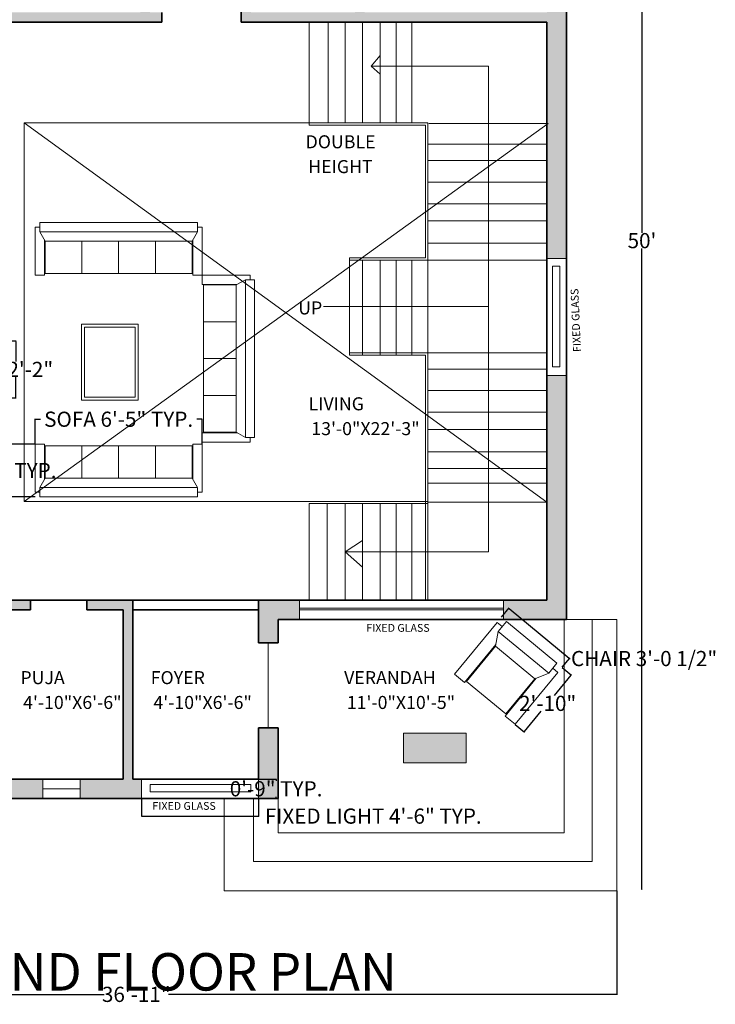
# Model space of a CAD drawing. Units: inches. Extents: x 136 to 672, y -412 to 279.
# Tile 3 of 6: x 351 to 672, y -412 to 42. Entities that reach past the tile are written whole.
import ezdxf

# ---------------------------------------------------------------- set-up
doc = ezdxf.new("R2010")
doc.units = ezdxf.units.IN
doc.header["$MEASUREMENT"] = 0
for name, color, linetype, lineweight in [('A-ANNO-DIMS', 12, 'Continuous', 18), ('A-ANNO-SYMB', 12, 'Continuous', 13), ('A-ANNO-TEXT', 7, 'Continuous', 18), ('A-AREA-IDEN', 7, 'Continuous', 18), ('A-DOOR', 4, 'Continuous', 18), ('A-FLOR-OPEN', 254, 'Continuous', 13), ('A-FLOR-STRS', 252, 'Continuous', 18), ('A-FURN-PATT', 143, 'Continuous', 9), ('A-WALL-PATT', 244, 'Continuous', 9), ('furniture', 252, 'Continuous', 18), ('walls', 253, 'Continuous', 35), ('windows', 171, 'Continuous', 18)]:
    doc.layers.add(name, color=color, linetype=linetype, lineweight=lineweight)
doc.styles.get("Standard").update_dxf_attribs({"font": 'arial.ttf'})
doc.dimstyles.get("Standard").update_dxf_attribs({"dimtxt": 7, "dimasz": 0.18, "dimexe": 0.18, "dimexo": 0.0625, "dimgap": 0.09, "dimtad": 0, "dimtih": 1, "dimtoh": 1, "dimzin": 0, "dimdsep": 46, "dimlunit": 3, "dimtxsty": 'Standard', "dimcen": 0.09, "dimadec": 0, "dimazin": 0, "dimtfac": 1, "dimtofl": 0, "dimtmove": 0, "dimatfit": 3, "dimfxl": 1, "dimtolj": 1, "dimtzin": 0, "dimarcsym": 0})

# ---------------------------------------------------------------- blocks, each defined once
blk = doc.blocks.new('FABRIC SOFA 1S')
at = {"layer": 'furniture'}
for p, q in [((0, -15.12), (0, 15.12)), ((6, 15.12), (0, 15.12)), ((3, 18.12), (34, 18.12)), ((3, 15.12), (3, 18.12)), ((6, -15.12), (6, 15.12)), ((12, 11.75), (6, 15.12)), ((34, 12.12), (34, 18.12)), ((11.33, 12.12), (34, 12.12)), ((6, -15.12), (12, -11.75)), ((11.33, -12.12), (34, -12.12)), ((34, -12.12), (34, -18.12)), ((6, -15.12), (0, -15.12)), ((3, -18.12), (3, -15.12)), ((3, -18.12), (34, -18.12))]:
    blk.add_line(p, q, dxfattribs=at)
blk.add_lwpolyline([(12, -11.75), (12, 11.75), (33, 11.75), (33, -11.75)], close=True, dxfattribs=at)
blk = doc.blocks.new('FABRIC SOFA 4S')
at = {"layer": 'furniture'}
for p, q in [((0, -51), (0, 51)), ((6, 51), (0, 51)), ((3, 54), (34, 54)), ((3, 51), (3, 54)), ((6, -51), (6, 51)), ((12, 47.63), (6, 51)), ((34, 48), (34, 54)), ((11.14, 48), (34, 48)), ((33, 23.81), (12, 23.81)), ((33, 0), (12, 0)), ((33, -23.81), (12, -23.81)), ((6, -51), (12, -47.63)), ((11.54, -48), (34, -48)), ((34, -48), (34, -54)), ((6, -51), (0, -51)), ((3, -54), (3, -51)), ((3, -54), (34, -54))]:
    blk.add_line(p, q, dxfattribs=at)
blk.add_lwpolyline([(12, -47.63), (12, 47.63), (33, 47.63), (33, -47.63)], close=True, dxfattribs=at)
blk = doc.blocks.new('*D20')
at = {"layer": 'A-ANNO-DIMS', "color": 0, "lineweight": -2, "transparency": 16777216}
for p, q in [((638.31, 239.56), (638.1, 239.56)), ((638.28, 239.38), (638.28, -56.02)), ((638.28, -358.76), (638.28, -63.35)), ((638.31, -358.94), (638.1, -358.94))]:
    blk.add_line(p, q, dxfattribs=at)
at = {"layer": 'A-ANNO-DIMS', "color": 0, "transparency": 16777216}
for points in [[(638.25, 239.38), (638.31, 239.38), (638.28, 239.56)], [(638.25, -358.76), (638.31, -358.76), (638.28, -358.94)]]:
    blk.add_solid(points, dxfattribs=at)
at = {"layer": 'Defpoints', "color": 0, "transparency": 16777216}
for p in [(638.37, 239.56), (638.28, -358.94), (638.37, -358.94)]:
    blk.add_point(p, dxfattribs=at)
at = {"layer": 'A-ANNO-DIMS', "color": 0, "transparency": 16777216, "insert": (638.28, -59.69), "char_height": 7, "attachment_point": 5}
blk.add_mtext("\\A1;50'", dxfattribs=at)
blk = doc.blocks.new('WIN-17')
for p, q in [((0, 9), (0, 0)), ((17.15, 9), (0, 9)), ((0, 9), (0, 4.5)), ((17.15, 0), (17.15, 9)), ((0, 4.5), (17.15, 4.5)), ((0, 0), (17.15, 0))]:
    blk.add_line(p, q)
blk = doc.blocks.new('WIN-FIXED-54')
for p, q in [((0, 9), (54.01, 9)), ((0, 0), (0, 9)), ((4.1, 6.5), (50.52, 6.5)), ((4.1, 3.12), (4.1, 6.5)), ((50.52, 6.5), (50.52, 3.12)), ((54.01, 9), (54.01, 0)), ((54.01, 0), (0, 0)), ((50.52, 3.12), (4.1, 3.12))]:
    blk.add_line(p, q)
blk = doc.blocks.new('*D35')
at = {"layer": 'A-ANNO-DIMS', "color": 0, "lineweight": -2, "transparency": 16777216}
for p, q in [((345.66, -105.96), (349.71, -105.96)), ((349.53, -106.14), (349.53, -115.47)), ((349.53, -132), (349.53, -122.68)), ((345.66, -132.18), (349.71, -132.18))]:
    blk.add_line(p, q, dxfattribs=at)
at = {"layer": 'A-ANNO-DIMS', "color": 0, "transparency": 16777216}
for points in [[(349.5, -106.14), (349.56, -106.14), (349.53, -105.96)], [(349.5, -132), (349.56, -132), (349.53, -132.18)]]:
    blk.add_solid(points, dxfattribs=at)
at = {"layer": 'Defpoints', "color": 0, "transparency": 16777216}
for p in [(345.6, -105.96), (349.53, -105.96), (345.6, -132.18)]:
    blk.add_point(p, dxfattribs=at)
at = {"layer": 'A-ANNO-DIMS', "color": 0, "transparency": 16777216, "insert": (349.53, -119.07), "char_height": 7, "attachment_point": 5}
blk.add_mtext('\\A1;TV 2\'-2"', dxfattribs=at)
blk = doc.blocks.new('*D37')
at = {"layer": 'A-ANNO-DIMS', "color": 0, "lineweight": -2, "transparency": 16777216}
for p, q in [((358.47, -153.53), (358.47, -141.86)), ((358.65, -142.04), (360.87, -142.04)), ((435.26, -142.04), (433.03, -142.04)), ((435.44, -153.53), (435.44, -141.86))]:
    blk.add_line(p, q, dxfattribs=at)
at = {"layer": 'A-ANNO-DIMS', "color": 0, "transparency": 16777216}
for points in [[(358.65, -142.01), (358.65, -142.07), (358.47, -142.04)], [(435.26, -142.01), (435.26, -142.07), (435.44, -142.04)]]:
    blk.add_solid(points, dxfattribs=at)
at = {"layer": 'Defpoints', "color": 0, "transparency": 16777216}
for p in [(435.44, -142.04), (358.47, -153.59), (435.44, -153.59)]:
    blk.add_point(p, dxfattribs=at)
at = {"layer": 'A-ANNO-DIMS', "color": 0, "transparency": 16777216, "insert": (396.95, -142.04), "char_height": 7, "attachment_point": 5}
blk.add_mtext('\\A1;SOFA 6\'-5" TYP.', dxfattribs=at)
blk = doc.blocks.new('*D38')
at = {"layer": 'A-ANNO-DIMS', "color": 0, "lineweight": -2, "transparency": 16777216}
for p, q in [((358.4, -153.59), (346.74, -153.59)), ((346.92, -153.77), (346.92, -162.04)), ((346.92, -177.64), (346.92, -169.37)), ((358.4, -177.82), (346.74, -177.82))]:
    blk.add_line(p, q, dxfattribs=at)
at = {"layer": 'A-ANNO-DIMS', "color": 0, "transparency": 16777216}
for points in [[(346.89, -153.77), (346.95, -153.77), (346.92, -153.59)], [(346.89, -177.64), (346.95, -177.64), (346.92, -177.82)]]:
    blk.add_solid(points, dxfattribs=at)
at = {"layer": 'Defpoints', "color": 0, "transparency": 16777216}
for p in [(346.92, -153.59), (358.47, -153.59), (358.47, -177.82)]:
    blk.add_point(p, dxfattribs=at)
at = {"layer": 'A-ANNO-DIMS', "color": 0, "transparency": 16777216, "insert": (346.92, -165.7), "char_height": 7, "attachment_point": 5}
blk.add_mtext('\\A1;2\'-0" TYP.', dxfattribs=at)
blk = doc.blocks.new('*D39')
at = {"layer": 'A-ANNO-DIMS', "color": 0, "lineweight": -2, "transparency": 16777216}
for p, q in [((573.47, -233.36), (577, -229.08)), ((577.03, -229.33), (604.72, -252.16)), ((601.44, -256.43), (604.97, -252.14)), ((604.86, -252.28), (605, -252.39)), ((605, -252.39), (605.18, -252.39))]:
    blk.add_line(p, q, dxfattribs=at)
at = {"layer": 'A-ANNO-DIMS', "color": 0, "transparency": 16777216}
for points in [[(577.05, -229.31), (577.01, -229.36), (576.89, -229.22)], [(604.74, -252.14), (604.7, -252.19), (604.86, -252.28)]]:
    blk.add_solid(points, dxfattribs=at)
at = {"layer": 'Defpoints', "color": 0, "transparency": 16777216}
for p in [(573.43, -233.41), (604.86, -252.28), (601.4, -256.47)]:
    blk.add_point(p, dxfattribs=at)
at = {"layer": 'A-ANNO-DIMS', "color": 0, "transparency": 16777216, "insert": (639.26, -252.39), "char_height": 7, "attachment_point": 5}
blk.add_mtext('\\A1;CHAIR 3\'-0 1/2"', dxfattribs=at)
blk = doc.blocks.new('*D40')
at = {"layer": 'A-ANNO-DIMS', "color": 0, "lineweight": -2, "transparency": 16777216}
for p, q in [((601.45, -256.51), (605.73, -260.05)), ((605.48, -260.07), (597.8, -269.39)), ((584.08, -286.03), (591.76, -276.71)), ((579.82, -282.75), (584.11, -286.28))]:
    blk.add_line(p, q, dxfattribs=at)
at = {"layer": 'A-ANNO-DIMS', "color": 0, "transparency": 16777216}
for points in [[(605.46, -260.05), (605.5, -260.09), (605.6, -259.93)], [(584.06, -286.01), (584.1, -286.05), (583.97, -286.17)]]:
    blk.add_solid(points, dxfattribs=at)
at = {"layer": 'Defpoints', "color": 0, "transparency": 16777216}
for p in [(601.4, -256.47), (579.77, -282.71), (583.97, -286.17)]:
    blk.add_point(p, dxfattribs=at)
at = {"layer": 'A-ANNO-DIMS', "color": 0, "transparency": 16777216, "insert": (594.78, -273.05), "char_height": 7, "attachment_point": 5}
blk.add_mtext('\\A1;2\'-10"', dxfattribs=at)
blk = doc.blocks.new('*D53')
at = {"layer": 'A-ANNO-DIMS', "color": 0, "lineweight": -2, "transparency": 16777216}
for p, q in [((407.45, -317), (407.45, -325.22)), ((461.46, -317), (461.46, -325.22)), ((407.63, -325.04), (461.28, -325.04)), ((461.46, -325.04), (461.64, -325.04))]:
    blk.add_line(p, q, dxfattribs=at)
at = {"layer": 'A-ANNO-DIMS', "color": 0, "transparency": 16777216}
for points in [[(407.63, -325.01), (407.63, -325.07), (407.45, -325.04)], [(461.28, -325.01), (461.28, -325.07), (461.46, -325.04)]]:
    blk.add_solid(points, dxfattribs=at)
at = {"layer": 'Defpoints', "color": 0, "transparency": 16777216}
for p in [(407.45, -316.94), (461.46, -316.94), (461.46, -325.04)]:
    blk.add_point(p, dxfattribs=at)
at = {"layer": 'A-ANNO-DIMS', "color": 0, "transparency": 16777216, "insert": (514.38, -325.04), "char_height": 7, "attachment_point": 5}
blk.add_mtext('\\A1;FIXED LIGHT 4\'-6" TYP.', dxfattribs=at)
blk = doc.blocks.new('*D54')
at = {"layer": 'A-ANNO-DIMS', "color": 0, "lineweight": -2, "transparency": 16777216}
for p, q in [((461.53, -307.94), (469.74, -307.94)), ((469.56, -308.12), (469.56, -308.77)), ((461.53, -316.94), (469.74, -316.94)), ((469.56, -316.76), (469.56, -316.1))]:
    blk.add_line(p, q, dxfattribs=at)
at = {"layer": 'A-ANNO-DIMS', "color": 0, "transparency": 16777216}
for points in [[(469.53, -308.12), (469.59, -308.12), (469.56, -307.94)], [(469.53, -316.76), (469.59, -316.76), (469.56, -316.94)]]:
    blk.add_solid(points, dxfattribs=at)
at = {"layer": 'Defpoints', "color": 0, "transparency": 16777216}
for p in [(461.46, -307.94), (469.56, -307.94), (461.46, -316.94)]:
    blk.add_point(p, dxfattribs=at)
at = {"layer": 'A-ANNO-DIMS', "color": 0, "transparency": 16777216, "insert": (469.56, -312.44), "char_height": 7, "attachment_point": 5}
blk.add_mtext('\\A1;0\'-9" TYP.', dxfattribs=at)
blk = doc.blocks.new('*D55')
at = {"layer": 'A-ANNO-DIMS', "color": 0, "lineweight": -2, "transparency": 16777216}
for p, q in [((183.46, -360.5), (183.46, -407.41)), ((626.7, -359.5), (626.7, -407.41)), ((183.64, -407.23), (390.25, -407.23)), ((626.52, -407.23), (419.91, -407.23))]:
    blk.add_line(p, q, dxfattribs=at)
at = {"layer": 'A-ANNO-DIMS', "color": 0, "transparency": 16777216}
for points in [[(183.64, -407.2), (183.64, -407.26), (183.46, -407.23)], [(626.52, -407.2), (626.52, -407.26), (626.7, -407.23)]]:
    blk.add_solid(points, dxfattribs=at)
at = {"layer": 'Defpoints', "color": 0, "transparency": 16777216}
for p in [(183.46, -360.44), (626.7, -359.44), (626.7, -407.23)]:
    blk.add_point(p, dxfattribs=at)
at = {"layer": 'A-ANNO-DIMS', "color": 0, "transparency": 16777216, "insert": (405.08, -407.23), "char_height": 7, "attachment_point": 5}
blk.add_mtext('\\A1;36\'-11"', dxfattribs=at)

msp = doc.modelspace()

# ---------------------------------------------------------------- hatches: boundary and pattern name
at = {"layer": 'A-FURN-PATT'}
h = msp.add_hatch(color=256, dxfattribs=at)
h.dxf.hatch_style = 1
h.paths.add_polyline_path([(557.179, -286.732), (528.261, -286.732), (528.261, -300.431), (557.179, -300.431)])
at = {"layer": 'A-WALL-PATT'}
h = msp.add_hatch(color=256, dxfattribs=at)
h.dxf.hatch_style = 1
h.paths.add_polyline_path([(255.026, 239.565), (183.463, 239.565), (183.463, 125.252), (187.963, 125.252), (192.463, 125.252), (192.463, 230.565), (255.024, 230.565), (255.025, 235.065)])
h.paths.add_polyline_path([(369.355, 239.565), (332.259, 239.565), (332.259, 230.565), (342.463, 230.565), (342.463, 104.521), (346.963, 104.521), (346.963, 230.565), (369.355, 230.565), (369.355, 235.065)])
h.paths.add_polyline_path([(603.463, 239.565), (385.627, 239.565), (385.627, 230.565), (406.963, 230.565), (406.963, 134.565), (371.802, 134.565), (371.802, 130.065), (406.963, 130.065), (406.963, 45.565), (346.963, 45.565), (346.963, 69.395), (342.463, 69.395), (342.463, 45.565), (332.733, 45.565), (332.733, 41.065), (416.87, 41.065), (416.87, 45.565), (411.463, 45.565), (411.463, 230.565), (594.463, 230.565), (594.463, 199.893), (598.963, 199.893), (603.463, 199.893)])
h.paths.add_polyline_path([(603.463, 145.845), (594.463, 145.845), (594.463, 98.065), (524.374, 98.065), (512.275, 97.948), (512.275, 98.065), (484.021, 98.065), (484.021, 93.565), (505.963, 93.565), (594.463, 93.565), (594.463, 80.073), (598.963, 80.073), (603.463, 80.073)], flags=17)
h.paths.add_polyline_path([(457.963, 98.065), (453.463, 98.065), (453.463, 41.065), (594.463, 41.065), (594.463, -67.933), (603.463, -67.933), (603.463, 63.801), (594.463, 63.801), (594.463, 45.565), (510.463, 45.565), (510.463, 65.243), (505.963, 65.243), (505.963, 45.565), (457.963, 45.565)])
h.paths.add_polyline_path([(192.463, 71.205), (183.463, 71.205), (183.463, 25.824), (192.463, 25.824), (192.463, 41.065), (296.463, 41.065), (296.463, 24.884), (300.963, 24.884), (300.963, 45.565), (192.463, 45.565)])
h.paths.add_polyline_path([(300.963, -6.935), (296.463, -6.935), (192.463, -6.935), (192.463, -11.435), (300.963, -11.435)])
h.paths.add_polyline_path([(192.463, 8.674), (183.463, 8.674), (183.463, -44.733), (187.963, -44.733), (192.463, -44.733)])
h.paths.add_polyline_path([(235.886, -349.935), (192.463, -349.935), (192.463, -358.935), (235.886, -358.935)])
h.paths.add_polyline_path([(345.463, -316.935), (361.986, -316.935), (361.986, -307.935), (340.963, -307.935), (340.963, -229.935), (356.354, -229.935), (356.354, -225.435), (336.463, -225.435), (336.463, -349.935), (300.655, -349.935), (300.655, -358.935), (345.463, -358.935)])
h.paths.add_polyline_path([(407.452, -307.935), (403.463, -307.935), (403.463, -225.435), (382.286, -225.435), (382.286, -229.935), (398.963, -229.935), (398.963, -307.935), (379.137, -307.935), (379.137, -316.935), (407.452, -316.935)])
h.paths.add_polyline_path([(470.463, -284.28), (461.463, -284.28), (461.463, -307.935), (461.463, -316.935), (470.463, -316.935)])
h.paths.add_polyline_path([(470.463, -234.435), (480.349, -234.435), (480.349, -225.435), (461.463, -225.435), (461.463, -245.135), (470.463, -245.135)])
h.paths.add_polyline_path([(603.463, -121.943), (594.463, -121.943), (594.463, -225.435), (574.368, -225.435), (574.368, -234.435), (603.463, -234.435)])
h.paths.add_polyline_path([(340.963, -75.678), (336.463, -75.678), (336.463, -168.061), (340.963, -168.061)])
h.paths.add_polyline_path([(468.637, 59.14), (510.671, 59.14), (510.671, 68.331), (468.637, 68.331)], flags=25)
h.paths.add_polyline_path([(192.463, -208.04), (183.463, -208.04), (183.463, -360.435), (192.463, -360.435)])
h.paths.add_polyline_path([(183.463, -153.992), (192.463, -153.992), (192.463, -98.781), (183.463, -98.781)])

# ---------------------------------------------------------------- linework, layer by layer
at = {"layer": 'A-ANNO-SYMB'}
for p, q in [((513.38, 20.691), (517.616, 25.629)), ((567.53, 20.691), (513.38, 20.691)), ((513.38, 20.691), (517.616, 17.058)), ((567.53, -203.204), (567.53, 20.691)), ((567.53, -90.03), (491.486, -90.03)), ((567.53, -90.03), (567.53, -90.03)), ((501.4, -203.204), (509.333, -197.906)), ((501.4, -203.204), (567.53, -203.204)), ((501.4, -203.204), (509.333, -210.301)), ((509.333, -210.301), (501.4, -203.204))]:
    msp.add_line(p, q, dxfattribs=at)
at = {"layer": 'A-DOOR'}
msp.add_line((465.963, -284.28), (465.963, -245.135), dxfattribs=at)
at = {"layer": 'A-FLOR-OPEN'}
for p, q in [((484.855, -5.321), (353.384, -5.321)), ((353.384, -5.321), (353.384, -179.904)), ((594.463, -180.25), (353.384, -5.321)), ((353.384, -179.904), (595.021, -5.62)), ((353.384, -179.904), (484.855, -179.904))]:
    msp.add_line(p, q, dxfattribs=at)
at = {"layer": 'A-FLOR-STRS'}
for p, q in [((484.855, 41.065), (484.855, -6.389)), ((493.589, -5.321), (493.589, 41.065)), ((501.4, -5.321), (501.4, 41.065)), ((509.333, -5.321), (509.333, 41.065)), ((517.616, -5.321), (517.616, 41.065)), ((524.879, -5.321), (524.879, 41.065)), ((532.105, -5.321), (532.105, 41.065)), ((484.855, -5.321), (539.481, -5.321)), ((484.855, -6.389), (538.413, -6.389)), ((538.413, -6.389), (538.413, -67.599)), ((539.481, -5.321), (539.481, -68.668)), ((540.039, -5.62), (595.021, -5.62)), ((539.481, -15.228), (594.463, -15.228)), ((539.481, -22.754), (594.463, -22.754)), ((539.481, -32.688), (594.463, -32.688)), ((539.481, -42.653), (594.463, -42.653)), ((539.481, -50.54), (594.463, -50.54)), ((539.481, -60.834), (594.463, -60.834)), ((538.413, -67.599), (503.376, -67.599)), ((503.376, -67.599), (503.376, -112.461)), ((539.481, -68.668), (503.376, -68.668)), ((509.333, -112.461), (509.333, -68.668)), ((517.616, -112.461), (517.616, -68.668)), ((524.879, -112.461), (524.879, -68.668)), ((532.105, -112.461), (532.105, -68.668)), ((539.481, -68.668), (539.481, -128.487)), ((539.481, -68.668), (594.463, -68.668)), ((503.376, -111.392), (539.481, -111.392)), ((503.376, -112.461), (538.413, -112.461)), ((538.413, -129.556), (538.413, -112.461)), ((539.481, -111.392), (594.463, -111.392)), ((539.481, -118.918), (594.463, -118.918)), ((538.413, -129.556), (538.413, -225.435)), ((539.481, -128.487), (539.481, -191.38)), ((539.481, -128.853), (594.463, -128.853)), ((539.481, -138.817), (594.463, -138.817)), ((539.481, -146.704), (594.463, -146.704)), ((539.481, -156.999), (594.463, -156.999)), ((539.481, -164.832), (594.463, -164.832)), ((539.481, -171.469), (594.463, -171.469)), ((539.481, -179.904), (484.855, -179.904)), ((484.855, -180.972), (484.855, -225.435)), ((539.481, -180.972), (484.855, -180.972)), ((493.117, -180.972), (493.117, -225.435)), ((501.4, -180.972), (501.4, -225.435)), ((509.333, -180.972), (509.333, -225.435)), ((517.616, -180.972), (517.616, -225.435)), ((524.879, -180.972), (524.879, -225.435)), ((532.105, -180.972), (532.105, -225.435)), ((539.481, -180.25), (594.463, -180.25)), ((539.481, -191.38), (539.481, -225.435)), ((602.463, -316.935), (602.463, -234.435)), ((616.434, -234.435), (603.463, -234.435)), ((615.298, -346.006), (615.298, -234.435)), ((626.698, -234.435), (616.434, -234.435)), ((626.698, -359.435), (626.698, -234.435)), ((445.61, -359.435), (445.61, -316.935)), ((459.132, -316.935), (459.132, -346.006)), ((470.463, -332.816), (470.463, -316.935)), ((602.463, -316.935), (602.463, -332.816)), ((602.463, -332.816), (470.463, -332.816)), ((459.132, -346.006), (615.298, -346.006)), ((470.463, -359.435), (445.61, -359.435)), ((470.463, -359.435), (603.463, -359.435)), ((603.463, -359.435), (626.698, -359.435))]:
    msp.add_line(p, q, dxfattribs=at)
at = {"layer": 'furniture'}
for p, q in [((379.895, -98.224), (405.915, -98.224)), ((379.895, -133.261), (379.895, -98.224)), ((381.221, -99.575), (404.55, -99.575)), ((381.221, -131.847), (381.221, -99.575)), ((404.55, -99.575), (404.55, -131.847)), ((405.915, -98.224), (405.915, -133.261)), ((405.915, -133.261), (379.895, -133.261)), ((404.55, -131.847), (381.221, -131.847)), ((528.261, -286.732), (557.179, -286.732)), ((528.261, -300.431), (528.261, -286.732)), ((557.179, -286.732), (557.179, -300.431)), ((557.179, -300.431), (528.261, -300.431))]:
    msp.add_line(p, q, dxfattribs=at)
at = {"layer": 'walls'}
for p, q in [((603.463, 239.565), (603.463, -234.435)), ((453.463, 98.065), (453.463, 41.065)), ((416.87, 45.565), (416.87, 41.065)), ((416.87, 41.065), (416.87, 45.565)), ((332.733, 41.065), (416.87, 41.065)), ((453.463, 41.065), (594.463, 41.065)), ((594.463, 41.065), (594.463, -225.435)), ((336.463, -225.435), (594.463, -225.435)), ((356.354, -225.435), (356.354, -229.935)), ((382.286, -225.435), (382.286, -229.935)), ((403.463, -307.935), (403.463, -225.435)), ((461.463, -245.135), (461.463, -225.435)), ((340.963, -229.935), (356.354, -229.935)), ((382.286, -229.935), (398.963, -229.935)), ((398.963, -307.935), (398.963, -229.935)), ((403.463, -229.935), (461.463, -229.935)), ((470.463, -234.435), (603.463, -234.435)), ((470.463, -245.135), (470.463, -234.435)), ((461.463, -245.135), (470.463, -245.135)), ((461.463, -307.935), (461.463, -284.28)), ((461.463, -284.28), (470.463, -284.28)), ((470.463, -316.935), (470.463, -284.28)), ((340.963, -307.935), (398.963, -307.935)), ((403.463, -307.935), (461.463, -307.935)), ((345.463, -316.935), (470.463, -316.935))]:
    msp.add_line(p, q, dxfattribs=at)
at = {"layer": 'windows'}
for p, q in [((480.349, -225.435), (480.349, -234.435)), ((574.368, -225.435), (480.349, -225.435)), ((480.349, -225.435), (480.349, -229.225)), ((574.368, -234.435), (574.368, -225.435)), ((480.349, -229.225), (574.368, -229.225)), ((574.368, -229.935), (480.349, -229.935)), ((574.368, -229.225), (574.368, -229.935)), ((480.349, -234.435), (574.368, -234.435))]:
    msp.add_line(p, q, dxfattribs=at)

# ---------------------------------------------------------------- block references
at = {"layer": 'furniture', "yscale": 0.7127038693416449, "zscale": 0.7127038693416449}
for p, xscale, rotation in [((396.952, -51.366), 0.7127038693416449, 270), ((459.67, -114.084), 0.7127038693416449, 180), ((396.952, -177.82), -0.7127038693416449, 270)]:
    msp.add_blockref('FABRIC SOFA 4S', p, dxfattribs=dict(at, xscale=xscale, rotation=rotation))
at = {"layer": 'furniture', "rotation": 230.4950403325632}
msp.add_blockref('FABRIC SOFA 1S', (587.415, -244.943), dxfattribs=at)
at = {"layer": 'windows', "rotation": 90}
msp.add_blockref('WIN-FIXED-54', (603.463, -121.943), dxfattribs=at)
at = {"layer": 'windows'}
for name, p in [('WIN-17', (361.986, -316.935)), ('WIN-FIXED-54', (407.452, -316.935))]:
    msp.add_blockref(name, p, dxfattribs=at)

# ---------------------------------------------------------------- texts
at = {"layer": 'A-ANNO-TEXT'}
msp.add_text('FIXED GLASS', height=3.59965, rotation=92.39712, dxfattribs=at).set_placement((610.148, -110.96))
for s, height, p in [('UP', 6, (479.756, -93.721)), ('FIXED GLASS', 3.59965, (511.154, -240.05)), ('FIXED GLASS', 3.59965, (412.52, -322.141)), ('GROUND FLOOR PLAN', 17.26909, (281.023, -405.489))]:
    msp.add_text(s, height=height, dxfattribs=at).set_placement(p)
at = {"layer": 'A-AREA-IDEN'}
for s, p in [('DOUBLE', (483.161, -17.11)), ('HEIGHT', (484.398, -28.557)), ('LIVING', (484.575, -137.924)), ('13\'-0"X22\'-3"', (485.813, -149.372)), ('PUJA', (351.647, -264.188)), ('FOYER', (411.745, -264.188)), ('VERANDAH', (500.94, -264.188)), ('4\'-10"X6\'-6"', (352.885, -275.636)), ('4\'-10"X6\'-6"', (412.982, -275.636)), ('11\'-0"X10\'-5"', (502.177, -275.636))]:
    msp.add_text(s, height=6, dxfattribs=at).set_placement(p)

# ---------------------------------------------------------------- dimensions: what is measured, and where the dimension line sits
at = {"layer": 'A-ANNO-DIMS'}
for base, p1, p2, angle, text, override, picture, middle in [((638.276, -358.935), (638.373, 239.565), (638.373, -358.935), 90, "50'", {"dimclrd": 0, "dimclre": 0, "dimclrt": 0}, '*D20', (638.276, -59.685)), ((349.532, -105.965), (345.6, -132.182), (345.6, -105.965), 90, 'TV <>', {"dimdec": 1, "dimlfac": 1, "dimrnd": 0, "dimzin": 1, "dimdsep": 46, "dimlunit": 4, "dimfrac": 2}, '*D35', (349.532, -119.073)), ((346.92, -153.588), (358.466, -177.82), (358.466, -153.588), 90, '<> TYP.', {"dimdec": 1, "dimlfac": 1, "dimrnd": 0, "dimzin": 1, "dimdsep": 46, "dimlunit": 4, "dimfrac": 2}, '*D38', (346.92, -165.704)), ((604.8589, -252.2779), (573.4304, -233.4131), (601.3998, -256.4733), 320.49504, 'CHAIR <>', {"dimdec": 1, "dimlfac": 1, "dimrnd": 0, "dimzin": 1, "dimdsep": 46, "dimlunit": 4, "dimfrac": 2}, '*D39', (639.2578, -252.3924)), ((469.564, -307.935), (461.463, -316.935), (461.463, -307.935), 90, '<> TYP.', {"dimdec": 1, "dimlfac": 1, "dimrnd": 0, "dimzin": 1, "dimdsep": 46, "dimlunit": 4, "dimfrac": 2}, '*D54', (469.564, -312.435))]:
    dim = msp.add_linear_dim(base=base, p1=p1, p2=p2, angle=angle, text=text, dimstyle='Standard', override=override, dxfattribs=at)
    dim.commit()
    dim.dimension.update_dxf_attribs({"geometry": picture, "text_midpoint": middle})
for base, p1, p2, text, picture, middle in [((435.438, -142.042), (358.466, -153.588), (435.438, -153.588), 'SOFA <> TYP.', '*D37', (396.952, -142.042)), ((461.463, -325.037), (407.452, -316.935), (461.463, -316.935), 'FIXED LIGHT <> TYP.', '*D53', (514.383, -325.037))]:
    dim = msp.add_linear_dim(base=base, p1=p1, p2=p2, text=text, dimstyle='Standard', override={"dimdec": 1, "dimlfac": 1, "dimrnd": 0, "dimzin": 1, "dimdsep": 46, "dimlunit": 4, "dimfrac": 2}, dxfattribs=at)
    dim.commit()
    dim.dimension.update_dxf_attribs({"geometry": picture, "text_midpoint": middle})
dim = msp.add_linear_dim(base=(583.966, -286.166), p1=(601.4, -256.473), p2=(579.771, -282.707), angle=230.49504, dimstyle='Standard', override={"dimdec": 1, "dimlfac": 1, "dimrnd": 0, "dimzin": 1, "dimdsep": 46, "dimlunit": 4, "dimfrac": 2}, dxfattribs=at)
dim.commit()
dim.dimension.update_dxf_attribs({"geometry": '*D40', "text_midpoint": (594.781, -273.049)})
dim = msp.add_linear_dim(base=(626.698, -407.228), p1=(183.463, -360.435), p2=(626.698, -359.435), dimstyle='Standard', override={"dimdec": 1, "dimlfac": 1, "dimrnd": 0, "dimzin": 1, "dimdsep": 46, "dimlunit": 4, "dimfrac": 2}, dxfattribs=at)
dim.commit()
dim.dimension.update_dxf_attribs({"geometry": '*D55', "text_midpoint": (405.08, -407.228)})

doc.saveas('drawing.dxf')
